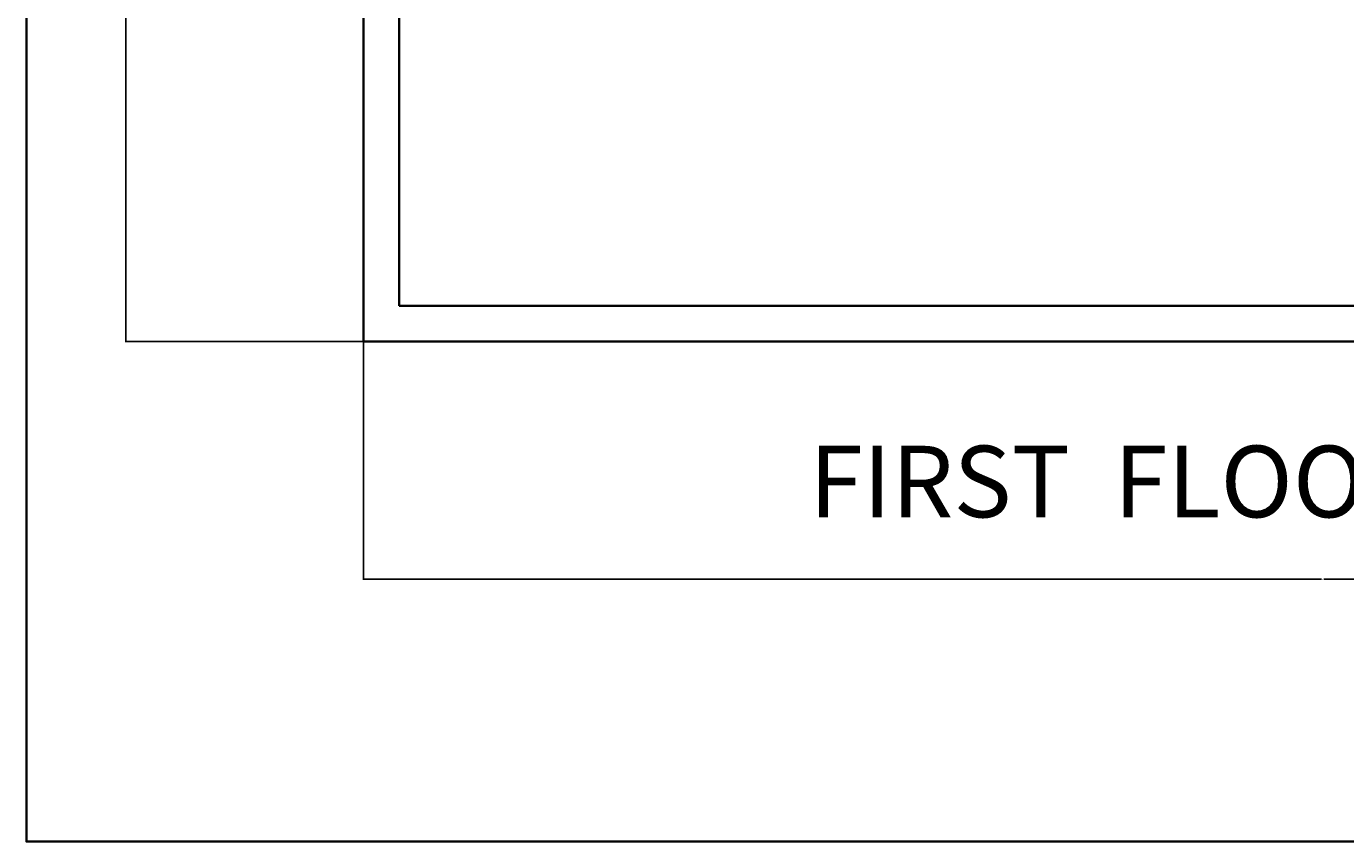
# Model space of a CAD drawing. Units: inches. Extents: x 2552 to 3217, y 1417 to 2737.
# Tile 1 of 25: x 2552 to 2885, y 1417 to 1622. Entities that reach past the tile are written whole.
import ezdxf

# ---------------------------------------------------------------- set-up
doc = ezdxf.new("R2010")
doc.units = ezdxf.units.IN
for name, color, linetype, lineweight in [('A-ANNO-DIMS', 2, 'Continuous', 18), ('A-ANNO-TEXT', 7, 'Continuous', 25), ('A-ANNO-TTLB', 7, 'Continuous', 35), ('A-WALL', 7, 'Continuous', 35)]:
    doc.layers.add(name, color=color, linetype=linetype, lineweight=lineweight)
doc.styles.get("Standard").update_dxf_attribs({"font": 'arial.ttf'})
doc.dimstyles.get("Standard").update_dxf_attribs({"dimtxt": 0.18, "dimasz": 0.18, "dimexe": 0.18, "dimexo": 0.0625, "dimgap": 0.09, "dimtad": 0, "dimtih": 1, "dimtoh": 1, "dimdec": 4, "dimzin": 0, "dimdsep": 46, "dimtxsty": 'Standard', "dimcen": 0.09, "dimadec": 0, "dimazin": 0, "dimtfac": 1, "dimtdec": 4, "dimtofl": 0, "dimtmove": 0, "dimatfit": 3, "dimfxl": 1, "dimtolj": 1, "dimtzin": 0, "dimarcsym": 0})

# ---------------------------------------------------------------- blocks, each defined once
blk = doc.blocks.new('*D49')
at = {"layer": 'A-ANNO-DIMS', "color": 0, "lineweight": -2, "transparency": 16777216}
for p, q in [((2637.35, 1542.45), (2637.35, 1482.53)), ((3120.35, 1542.45), (3120.35, 1482.53)), ((2637.53, 1482.71), (2878.56, 1482.71)), ((3120.17, 1482.71), (2879.15, 1482.71))]:
    blk.add_line(p, q, dxfattribs=at)
at = {"layer": 'A-ANNO-DIMS', "color": 0, "transparency": 16777216}
for points in [[(2637.53, 1482.74), (2637.53, 1482.68), (2637.35, 1482.71)], [(3120.17, 1482.74), (3120.17, 1482.68), (3120.35, 1482.71)]]:
    blk.add_solid(points, dxfattribs=at)
at = {"layer": 'Defpoints', "color": 0, "transparency": 16777216}
for p in [(2637.35, 1542.51), (3120.35, 1542.51), (3120.35, 1482.71)]:
    blk.add_point(p, dxfattribs=at)
at = {"layer": 'A-ANNO-DIMS', "color": 0, "transparency": 16777216, "insert": (2878.85, 1482.71), "char_height": 0.18, "attachment_point": 5}
blk.add_mtext('\\A1;483', dxfattribs=at)
blk = doc.blocks.new('*D50')
at = {"layer": 'A-ANNO-DIMS', "color": 0, "lineweight": -2, "transparency": 16777216}
for p, q in [((2637.29, 2649.51), (2577.37, 2649.51)), ((2577.55, 2649.33), (2577.55, 2096.19)), ((2577.55, 1542.69), (2577.55, 2095.83)), ((2637.29, 1542.51), (2577.37, 1542.51))]:
    blk.add_line(p, q, dxfattribs=at)
at = {"layer": 'A-ANNO-DIMS', "color": 0, "transparency": 16777216}
for points in [[(2577.52, 2649.33), (2577.58, 2649.33), (2577.55, 2649.51)], [(2577.52, 1542.69), (2577.58, 1542.69), (2577.55, 1542.51)]]:
    blk.add_solid(points, dxfattribs=at)
at = {"layer": 'Defpoints', "color": 0, "transparency": 16777216}
for p in [(2577.55, 2649.51), (2637.35, 2649.51), (2637.35, 1542.51)]:
    blk.add_point(p, dxfattribs=at)
at = {"layer": 'A-ANNO-DIMS', "color": 0, "transparency": 16777216, "insert": (2577.55, 2096.01), "char_height": 0.18, "attachment_point": 5}
blk.add_mtext('\\A1;1107', dxfattribs=at)
blk = doc.blocks.new('*D64')
at = {"layer": 'A-ANNO-DIMS', "color": 0, "lineweight": -2, "transparency": 16777216}
for p, q in [((2646.35, 1551.58), (2646.35, 2709.49)), ((2646.53, 2709.31), (2802.77, 2709.31)), ((2959.93, 2709.31), (2803.69, 2709.31)), ((2960.11, 1551.58), (2960.11, 2709.49))]:
    blk.add_line(p, q, dxfattribs=at)
at = {"layer": 'A-ANNO-DIMS', "color": 0, "transparency": 16777216}
for points in [[(2646.53, 2709.34), (2646.53, 2709.28), (2646.35, 2709.31)], [(2959.93, 2709.34), (2959.93, 2709.28), (2960.11, 2709.31)]]:
    blk.add_solid(points, dxfattribs=at)
at = {"layer": 'Defpoints', "color": 0, "transparency": 16777216}
for p in [(2960.11, 2709.31), (2646.35, 1551.51), (2960.11, 1551.51)]:
    blk.add_point(p, dxfattribs=at)
at = {"layer": 'A-ANNO-DIMS', "color": 0, "transparency": 16777216, "insert": (2803.23, 2709.31), "char_height": 0.18, "attachment_point": 5}
blk.add_mtext('\\A1;313.76', dxfattribs=at)

msp = doc.modelspace()

# ---------------------------------------------------------------- linework, layer by layer
at = {"layer": 'A-ANNO-TTLB'}
msp.add_lwpolyline([(2552.473, 2736.5692), (3216.7862, 2736.5692), (3216.7862, 1416.6914), (2552.473, 1416.6914)], close=True, dxfattribs=at)
at = {"layer": 'A-WALL'}
for p, q in [((2637.3535, 1542.5125), (2637.3535, 1626.5125)), ((2646.3535, 1551.5125), (2646.3535, 1626.5125)), ((3111.3535, 1551.5125), (2646.3535, 1551.5125)), ((2938.5018, 1542.5125), (2637.3535, 1542.5125))]:
    msp.add_line(p, q, dxfattribs=at)

# ---------------------------------------------------------------- texts
at = {"layer": 'A-ANNO-TEXT', "insert": (2749.5428, 1516.3052), "char_height": 18, "attachment_point": 1}
msp.add_mtext_dynamic_manual_height_columns('{FIRST  FLOOR  PLAN}', width=366.4635, gutter_width=12.5, heights=[0], dxfattribs=at)

# ---------------------------------------------------------------- dimensions: what is measured, and where the dimension line sits
at = {"layer": 'A-ANNO-DIMS'}
for base, p1, p2, override, picture, middle in [((2960.1089, 2709.3125), (2646.3535, 1551.5125), (2960.1089, 1551.5125), {"dimdec": 2, "dimlfac": 1, "dimrnd": 0, "dimzin": 0, "dimdsep": 46, "dimlunit": 2}, '*D64', (2803.2312, 2709.3125)), ((3120.3535, 1482.7125), (2637.3535, 1542.5125), (3120.3535, 1542.5125), {"dimdec": 0, "dimlfac": 1, "dimrnd": 0, "dimzin": 0, "dimdsep": 46, "dimlunit": 2}, '*D49', (2878.8535, 1482.7125))]:
    dim = msp.add_linear_dim(base=base, p1=p1, p2=p2, dimstyle='Standard', override=override, dxfattribs=at)
    dim.commit()
    dim.dimension.update_dxf_attribs({"geometry": picture, "text_midpoint": middle})
dim = msp.add_linear_dim(base=(2577.5535, 2649.5125), p1=(2637.3535, 1542.5125), p2=(2637.3535, 2649.5125), angle=90, dimstyle='Standard', override={"dimdec": 0, "dimlfac": 1, "dimrnd": 0, "dimzin": 0, "dimdsep": 46, "dimlunit": 2}, dxfattribs=at)
dim.commit()
dim.dimension.update_dxf_attribs({"geometry": '*D50', "text_midpoint": (2577.5535, 2096.0125)})

doc.saveas('drawing.dxf')
